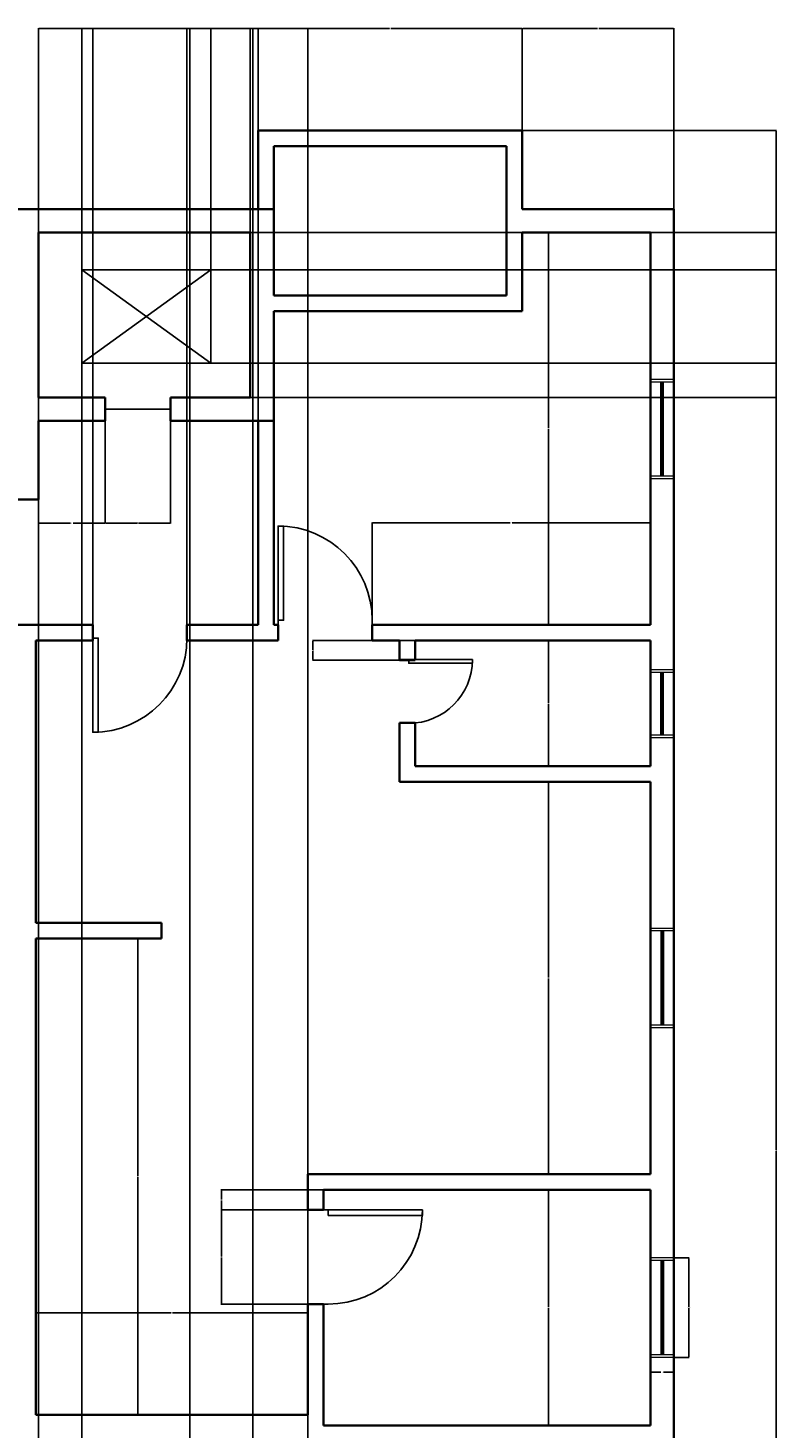
# Model space of a CAD drawing. Units: inches. Extents: x -7288 to -6705, y 7169 to 8028.
# Tile 5 of 5: x -6992 to -6705, y 7493 to 8028. Entities that reach past the tile are written whole.
import ezdxf

# ---------------------------------------------------------------- set-up
doc = ezdxf.new("R2010")
doc.units = ezdxf.units.IN
for name, color, linetype, lineweight in [('A-ANNO-DIMS', 2, 'Continuous', 18), ('A-DOOR', 3, 'Continuous', 25), ('A-FLOR-EVTR', 4, 'Continuous', 25), ('A-GLAZ', 2, 'Continuous', 18), ('A-WALL', 1, 'Continuous', 35)]:
    doc.layers.add(name, color=color, linetype=linetype, lineweight=lineweight)
doc.styles.get("Standard").update_dxf_attribs({"font": 'arial.ttf'})
doc.dimstyles.get("Standard").update_dxf_attribs({"dimtxt": 0.18, "dimasz": 0.18, "dimexe": 0.18, "dimexo": 0.0625, "dimgap": 0.09, "dimtad": 0, "dimtih": 1, "dimtoh": 1, "dimdec": 4, "dimzin": 0, "dimdsep": 46, "dimtxsty": 'Standard', "dimcen": 0.09, "dimadec": 0, "dimazin": 0, "dimtfac": 1, "dimtdec": 4, "dimtofl": 0, "dimtmove": 0, "dimatfit": 3, "dimfxl": 1, "dimtolj": 1, "dimtzin": 0, "dimarcsym": 0})

# ---------------------------------------------------------------- blocks, each defined once
blk = doc.blocks.new('*U8')
for p, q in [((0, 0), (0, -100)), ((750, 0), (750, -100))]:
    blk.add_line(p, q)
blk.add_lwpolyline([(0, 0), (0, 750), (43.75, 750), (43.75, 0)], close=True)
blk.add_arc((0, 0), 750, 0, 90)
blk = doc.blocks.new('WIN-36IN-WALL9')
for p, q in [((0, 38), (9, 38)), ((0, 37), (9, 37)), ((4, 1), (4, 37)), ((4.5, 1), (4.5, 37)), ((5, 1), (5, 37)), ((0, 1), (9, 1)), ((0, 0), (9, 0))]:
    blk.add_line(p, q)
blk = doc.blocks.new('WIN-24IN-WALL9')
for p, q in [((0, 26), (9, 26)), ((0, 25), (9, 25)), ((4, 1), (4, 25)), ((4.5, 1), (4.5, 25)), ((5, 1), (5, 25)), ((0, 1), (9, 1)), ((0, 0), (9, 0))]:
    blk.add_line(p, q)
blk = doc.blocks.new('*D87')
at = {"layer": 'A-ANNO-DIMS', "color": 0, "lineweight": -2, "transparency": 16777216}
for p, q in [((-6744.78, 7557.53), (-6738.96, 7557.53)), ((-6739.14, 7557.35), (-6739.14, 7538.71)), ((-6739.14, 7519.71), (-6739.14, 7538.35)), ((-6744.78, 7519.53), (-6738.96, 7519.53))]:
    blk.add_line(p, q, dxfattribs=at)
at = {"layer": 'A-ANNO-DIMS', "color": 0, "transparency": 16777216}
for points in [[(-6739.17, 7557.35), (-6739.11, 7557.35), (-6739.14, 7557.53)], [(-6739.17, 7519.71), (-6739.11, 7519.71), (-6739.14, 7519.53)]]:
    blk.add_solid(points, dxfattribs=at)
at = {"layer": 'Defpoints', "color": 0, "transparency": 16777216}
for p in [(-6744.84, 7557.53), (-6744.84, 7519.53), (-6739.14, 7519.53)]:
    blk.add_point(p, dxfattribs=at)
at = {"layer": 'A-ANNO-DIMS', "color": 0, "transparency": 16777216, "insert": (-6739.14, 7538.53), "char_height": 0.18, "attachment_point": 5}
blk.add_mtext('\\A1;W1 38 TYP.', dxfattribs=at)
blk = doc.blocks.new('*D88')
at = {"layer": 'A-ANNO-DIMS', "color": 0, "lineweight": -2, "transparency": 16777216}
for p, q in [((-6753.84, 7519.47), (-6753.84, 7513.65)), ((-6744.84, 7519.47), (-6744.84, 7513.65)), ((-6753.66, 7513.83), (-6749.8, 7513.83)), ((-6745.02, 7513.83), (-6748.88, 7513.83))]:
    blk.add_line(p, q, dxfattribs=at)
at = {"layer": 'A-ANNO-DIMS', "color": 0, "transparency": 16777216}
for points in [[(-6753.66, 7513.86), (-6753.66, 7513.8), (-6753.84, 7513.83)], [(-6745.02, 7513.86), (-6745.02, 7513.8), (-6744.84, 7513.83)]]:
    blk.add_solid(points, dxfattribs=at)
at = {"layer": 'Defpoints', "color": 0, "transparency": 16777216}
for p in [(-6753.84, 7519.53), (-6744.84, 7519.53), (-6753.84, 7513.83)]:
    blk.add_point(p, dxfattribs=at)
at = {"layer": 'A-ANNO-DIMS', "color": 0, "transparency": 16777216, "insert": (-6749.34, 7513.83), "char_height": 0.18, "attachment_point": 5}
blk.add_mtext('\\A1;9 TYP.', dxfattribs=at)
blk = doc.blocks.new('*D94')
at = {"layer": 'A-ANNO-DIMS', "color": 0, "lineweight": -2, "transparency": 16777216}
for p, q in [((-6802.78, 7988.53), (-6705.63, 7988.53)), ((-6705.81, 7988.35), (-6705.81, 7598.71)), ((-6705.81, 7208.71), (-6705.81, 7598.35)), ((-6744.78, 7208.53), (-6705.63, 7208.53))]:
    blk.add_line(p, q, dxfattribs=at)
at = {"layer": 'A-ANNO-DIMS', "color": 0, "transparency": 16777216}
for points in [[(-6705.84, 7988.35), (-6705.78, 7988.35), (-6705.81, 7988.53)], [(-6705.84, 7208.71), (-6705.78, 7208.71), (-6705.81, 7208.53)]]:
    blk.add_solid(points, dxfattribs=at)
at = {"layer": 'Defpoints', "color": 0, "transparency": 16777216}
for p in [(-6802.84, 7988.53), (-6705.81, 7988.53), (-6744.84, 7208.53)]:
    blk.add_point(p, dxfattribs=at)
at = {"layer": 'A-ANNO-DIMS', "color": 0, "transparency": 16777216, "insert": (-6705.81, 7598.53), "char_height": 0.18, "attachment_point": 5}
blk.add_mtext('\\A1;780', dxfattribs=at)
blk = doc.blocks.new('*D97')
at = {"layer": 'A-ANNO-DIMS', "color": 0, "lineweight": -2, "transparency": 16777216}
for p, q in [((-6903.84, 7988.59), (-6903.84, 8027.74)), ((-6903.66, 8027.56), (-6853.6, 8027.56)), ((-6803.02, 8027.56), (-6853.08, 8027.56)), ((-6802.84, 7988.59), (-6802.84, 8027.74))]:
    blk.add_line(p, q, dxfattribs=at)
at = {"layer": 'A-ANNO-DIMS', "color": 0, "transparency": 16777216}
for points in [[(-6903.66, 8027.59), (-6903.66, 8027.53), (-6903.84, 8027.56)], [(-6803.02, 8027.59), (-6803.02, 8027.53), (-6802.84, 8027.56)]]:
    blk.add_solid(points, dxfattribs=at)
at = {"layer": 'Defpoints', "color": 0, "transparency": 16777216}
for p in [(-6802.84, 8027.56), (-6903.84, 7988.53), (-6802.84, 7988.53)]:
    blk.add_point(p, dxfattribs=at)
at = {"layer": 'A-ANNO-DIMS', "color": 0, "transparency": 16777216, "insert": (-6853.34, 8027.56), "char_height": 0.18, "attachment_point": 5}
blk.add_mtext('\\A1;101', dxfattribs=at)
blk = doc.blocks.new('*D98')
at = {"layer": 'A-ANNO-DIMS', "color": 0, "lineweight": -2, "transparency": 16777216}
for p, q in [((-6802.84, 7988.59), (-6802.84, 8027.74)), ((-6802.66, 8027.56), (-6774.06, 8027.56)), ((-6745.02, 8027.56), (-6773.62, 8027.56)), ((-6744.84, 7958.59), (-6744.84, 8027.74))]:
    blk.add_line(p, q, dxfattribs=at)
at = {"layer": 'A-ANNO-DIMS', "color": 0, "transparency": 16777216}
for points in [[(-6802.66, 8027.59), (-6802.66, 8027.53), (-6802.84, 8027.56)], [(-6745.02, 8027.59), (-6745.02, 8027.53), (-6744.84, 8027.56)]]:
    blk.add_solid(points, dxfattribs=at)
at = {"layer": 'Defpoints', "color": 0, "transparency": 16777216}
for p in [(-6744.84, 8027.56), (-6802.84, 7988.53), (-6744.84, 7958.53)]:
    blk.add_point(p, dxfattribs=at)
at = {"layer": 'A-ANNO-DIMS', "color": 0, "transparency": 16777216, "insert": (-6773.84, 8027.56), "char_height": 0.18, "attachment_point": 5}
blk.add_mtext('\\A1;58', dxfattribs=at)
blk = doc.blocks.new('*D104')
at = {"layer": 'A-ANNO-DIMS', "color": 0, "lineweight": -2, "transparency": 16777216}
for p, q in [((-6987.84, 7949.59), (-6987.84, 8027.74)), ((-6987.66, 8027.56), (-6947.54, 8027.56)), ((-6907.02, 8027.56), (-6947.14, 8027.56)), ((-6906.84, 7949.59), (-6906.84, 8027.74))]:
    blk.add_line(p, q, dxfattribs=at)
at = {"layer": 'A-ANNO-DIMS', "color": 0, "transparency": 16777216}
for points in [[(-6987.66, 8027.59), (-6987.66, 8027.53), (-6987.84, 8027.56)], [(-6907.02, 8027.59), (-6907.02, 8027.53), (-6906.84, 8027.56)]]:
    blk.add_solid(points, dxfattribs=at)
at = {"layer": 'Defpoints', "color": 0, "transparency": 16777216}
for p in [(-6906.84, 8027.56), (-6987.84, 7949.53), (-6906.84, 7949.53)]:
    blk.add_point(p, dxfattribs=at)
at = {"layer": 'A-ANNO-DIMS', "color": 0, "transparency": 16777216, "insert": (-6947.34, 8027.56), "char_height": 0.18, "attachment_point": 5}
blk.add_mtext('\\A1;81', dxfattribs=at)
blk = doc.blocks.new('*D105')
at = {"layer": 'A-ANNO-DIMS', "color": 0, "lineweight": -2, "transparency": 16777216}
for p, q in [((-6906.78, 7949.53), (-6705.63, 7949.53)), ((-6705.81, 7949.35), (-6705.81, 7918.21)), ((-6705.81, 7886.71), (-6705.81, 7917.85)), ((-6906.78, 7886.53), (-6705.63, 7886.53))]:
    blk.add_line(p, q, dxfattribs=at)
at = {"layer": 'A-ANNO-DIMS', "color": 0, "transparency": 16777216}
for points in [[(-6705.84, 7949.35), (-6705.78, 7949.35), (-6705.81, 7949.53)], [(-6705.84, 7886.71), (-6705.78, 7886.71), (-6705.81, 7886.53)]]:
    blk.add_solid(points, dxfattribs=at)
at = {"layer": 'Defpoints', "color": 0, "transparency": 16777216}
for p in [(-6906.84, 7949.53), (-6705.81, 7949.53), (-6906.84, 7886.53)]:
    blk.add_point(p, dxfattribs=at)
at = {"layer": 'A-ANNO-DIMS', "color": 0, "transparency": 16777216, "insert": (-6705.81, 7918.03), "char_height": 0.18, "attachment_point": 5}
blk.add_mtext('\\A1;63', dxfattribs=at)
blk = doc.blocks.new('*D109')
at = {"layer": 'A-ANNO-DIMS', "color": 0, "lineweight": -2, "transparency": 16777216}
for p, q in [((-6962.28, 7877.47), (-6962.28, 7838.32)), ((-6937.29, 7877.47), (-6937.29, 7838.32)), ((-6962.1, 7838.5), (-6950.01, 7838.5)), ((-6937.47, 7838.5), (-6949.56, 7838.5))]:
    blk.add_line(p, q, dxfattribs=at)
at = {"layer": 'A-ANNO-DIMS', "color": 0, "transparency": 16777216}
for points in [[(-6962.1, 7838.53), (-6962.1, 7838.47), (-6962.28, 7838.5)], [(-6937.47, 7838.53), (-6937.47, 7838.47), (-6937.29, 7838.5)]]:
    blk.add_solid(points, dxfattribs=at)
at = {"layer": 'Defpoints', "color": 0, "transparency": 16777216}
for p in [(-6962.28, 7877.53), (-6937.29, 7877.53), (-6962.28, 7838.5)]:
    blk.add_point(p, dxfattribs=at)
at = {"layer": 'A-ANNO-DIMS', "color": 0, "transparency": 16777216, "insert": (-6949.78, 7838.5), "char_height": 0.18, "attachment_point": 5}
blk.add_mtext('\\A1;25', dxfattribs=at)
blk = doc.blocks.new('*D113')
at = {"layer": 'A-ANNO-DIMS', "color": 0, "lineweight": -2, "transparency": 16777216}
for p, q in [((-6971.26, 7935.37), (-6971.26, 8027.74)), ((-6971.08, 8027.56), (-6947.02, 8027.56)), ((-6922.15, 8027.56), (-6946.22, 8027.56)), ((-6921.97, 7935.37), (-6921.97, 8027.74))]:
    blk.add_line(p, q, dxfattribs=at)
at = {"layer": 'A-ANNO-DIMS', "color": 0, "transparency": 16777216}
for points in [[(-6971.08, 8027.59), (-6971.08, 8027.53), (-6971.26, 8027.56)], [(-6922.15, 8027.59), (-6922.15, 8027.53), (-6921.97, 8027.56)]]:
    blk.add_solid(points, dxfattribs=at)
at = {"layer": 'Defpoints', "color": 0, "transparency": 16777216}
for p in [(-6921.97, 8027.56), (-6971.26, 7935.31), (-6921.97, 7935.31)]:
    blk.add_point(p, dxfattribs=at)
at = {"layer": 'A-ANNO-DIMS', "color": 0, "transparency": 16777216, "insert": (-6946.62, 8027.56), "char_height": 0.18, "attachment_point": 5}
blk.add_mtext('\\A1;49.29', dxfattribs=at)
blk = doc.blocks.new('*D114')
at = {"layer": 'A-ANNO-DIMS', "color": 0, "lineweight": -2, "transparency": 16777216}
for p, q in [((-6921.91, 7935.31), (-6705.63, 7935.31)), ((-6705.81, 7935.13), (-6705.81, 7917.61)), ((-6705.81, 7899.73), (-6705.81, 7917.25)), ((-6921.91, 7899.55), (-6705.63, 7899.55))]:
    blk.add_line(p, q, dxfattribs=at)
at = {"layer": 'A-ANNO-DIMS', "color": 0, "transparency": 16777216}
for points in [[(-6705.84, 7935.13), (-6705.78, 7935.13), (-6705.81, 7935.31)], [(-6705.84, 7899.73), (-6705.78, 7899.73), (-6705.81, 7899.55)]]:
    blk.add_solid(points, dxfattribs=at)
at = {"layer": 'Defpoints', "color": 0, "transparency": 16777216}
for p in [(-6921.97, 7935.31), (-6705.81, 7935.31), (-6921.97, 7899.55)]:
    blk.add_point(p, dxfattribs=at)
at = {"layer": 'A-ANNO-DIMS', "color": 0, "transparency": 16777216, "insert": (-6705.81, 7917.43), "char_height": 0.18, "attachment_point": 5}
blk.add_mtext('\\A1;35.76', dxfattribs=at)
blk = doc.blocks.new('*D115')
at = {"layer": 'A-ANNO-DIMS', "color": 0, "lineweight": -2, "transparency": 16777216}
for p, q in [((-6971.26, 7899.49), (-6971.26, 7169.32)), ((-6987.84, 7886.47), (-6987.84, 7169.32)), ((-6987.66, 7169.5), (-6980.01, 7169.5)), ((-6971.44, 7169.5), (-6979.1, 7169.5))]:
    blk.add_line(p, q, dxfattribs=at)
at = {"layer": 'A-ANNO-DIMS', "color": 0, "transparency": 16777216}
for points in [[(-6987.66, 7169.53), (-6987.66, 7169.47), (-6987.84, 7169.5)], [(-6971.44, 7169.53), (-6971.44, 7169.47), (-6971.26, 7169.5)]]:
    blk.add_solid(points, dxfattribs=at)
at = {"layer": 'Defpoints', "color": 0, "transparency": 16777216}
for p in [(-6971.26, 7899.55), (-6987.84, 7886.53), (-6971.26, 7169.5)]:
    blk.add_point(p, dxfattribs=at)
at = {"layer": 'A-ANNO-DIMS', "color": 0, "transparency": 16777216, "insert": (-6979.55, 7169.5), "char_height": 0.18, "attachment_point": 5}
blk.add_mtext('\\A1;16.578', dxfattribs=at)
blk = doc.blocks.new('*D116')
at = {"layer": 'A-ANNO-DIMS', "color": 0, "lineweight": -2, "transparency": 16777216}
for p, q in [((-6987.78, 7949.53), (-6705.63, 7949.53)), ((-6705.81, 7949.35), (-6705.81, 7942.6)), ((-6705.81, 7935.49), (-6705.81, 7942.24)), ((-6971.2, 7935.31), (-6705.63, 7935.31))]:
    blk.add_line(p, q, dxfattribs=at)
at = {"layer": 'A-ANNO-DIMS', "color": 0, "transparency": 16777216}
for points in [[(-6705.84, 7949.35), (-6705.78, 7949.35), (-6705.81, 7949.53)], [(-6705.84, 7935.49), (-6705.78, 7935.49), (-6705.81, 7935.31)]]:
    blk.add_solid(points, dxfattribs=at)
at = {"layer": 'Defpoints', "color": 0, "transparency": 16777216}
for p in [(-6987.84, 7949.53), (-6705.81, 7949.53), (-6971.26, 7935.31)]:
    blk.add_point(p, dxfattribs=at)
at = {"layer": 'A-ANNO-DIMS', "color": 0, "transparency": 16777216, "insert": (-6705.81, 7942.42), "char_height": 0.18, "attachment_point": 5}
blk.add_mtext('\\A1;14.222', dxfattribs=at)
blk = doc.blocks.new('*D117')
at = {"layer": 'A-ANNO-DIMS', "color": 0, "lineweight": -2, "transparency": 16777216}
for p, q in [((-6987.84, 7877.47), (-6987.84, 7838.32)), ((-6962.28, 7877.47), (-6962.28, 7838.32)), ((-6987.66, 7838.5), (-6975.53, 7838.5)), ((-6962.46, 7838.5), (-6974.6, 7838.5))]:
    blk.add_line(p, q, dxfattribs=at)
at = {"layer": 'A-ANNO-DIMS', "color": 0, "transparency": 16777216}
for points in [[(-6987.66, 7838.53), (-6987.66, 7838.47), (-6987.84, 7838.5)], [(-6962.46, 7838.53), (-6962.46, 7838.47), (-6962.28, 7838.5)]]:
    blk.add_solid(points, dxfattribs=at)
at = {"layer": 'Defpoints', "color": 0, "transparency": 16777216}
for p in [(-6987.84, 7877.53), (-6962.28, 7877.53), (-6987.84, 7838.5)]:
    blk.add_point(p, dxfattribs=at)
at = {"layer": 'A-ANNO-DIMS', "color": 0, "transparency": 16777216, "insert": (-6975.06, 7838.5), "char_height": 0.18, "attachment_point": 5}
blk.add_mtext('\\A1;25.556', dxfattribs=at)
blk = doc.blocks.new('*D120')
at = {"layer": 'A-ANNO-DIMS', "color": 0, "lineweight": -2, "transparency": 16777216}
for p, q in [((-6967.07, 7799.59), (-6967.07, 8027.74)), ((-6966.89, 8027.56), (-6949.29, 8027.56)), ((-6931.25, 8027.56), (-6948.85, 8027.56)), ((-6931.07, 7799.59), (-6931.07, 8027.74))]:
    blk.add_line(p, q, dxfattribs=at)
at = {"layer": 'A-ANNO-DIMS', "color": 0, "transparency": 16777216}
for points in [[(-6966.89, 8027.59), (-6966.89, 8027.53), (-6967.07, 8027.56)], [(-6931.25, 8027.59), (-6931.25, 8027.53), (-6931.07, 8027.56)]]:
    blk.add_solid(points, dxfattribs=at)
at = {"layer": 'Defpoints', "color": 0, "transparency": 16777216}
for p in [(-6931.07, 8027.56), (-6967.07, 7799.53), (-6931.07, 7799.53)]:
    blk.add_point(p, dxfattribs=at)
at = {"layer": 'A-ANNO-DIMS', "color": 0, "transparency": 16777216, "insert": (-6949.07, 8027.56), "char_height": 0.18, "attachment_point": 5}
blk.add_mtext('\\A1;36', dxfattribs=at)
blk = doc.blocks.new('*D121')
at = {"layer": 'A-ANNO-DIMS', "color": 0, "lineweight": -2, "transparency": 16777216}
for p, q in [((-6931.07, 7799.59), (-6931.07, 8027.74)), ((-6930.89, 8027.56), (-6917.85, 8027.56)), ((-6904.02, 8027.56), (-6917.06, 8027.56)), ((-6903.84, 7799.59), (-6903.84, 8027.74))]:
    blk.add_line(p, q, dxfattribs=at)
at = {"layer": 'A-ANNO-DIMS', "color": 0, "transparency": 16777216}
for points in [[(-6930.89, 8027.59), (-6930.89, 8027.53), (-6931.07, 8027.56)], [(-6904.02, 8027.59), (-6904.02, 8027.53), (-6903.84, 8027.56)]]:
    blk.add_solid(points, dxfattribs=at)
at = {"layer": 'Defpoints', "color": 0, "transparency": 16777216}
for p in [(-6903.84, 8027.56), (-6931.07, 7799.53), (-6903.84, 7799.53)]:
    blk.add_point(p, dxfattribs=at)
at = {"layer": 'A-ANNO-DIMS', "color": 0, "transparency": 16777216, "insert": (-6917.45, 8027.56), "char_height": 0.18, "attachment_point": 5}
blk.add_mtext('\\A1;27.23', dxfattribs=at)
blk = doc.blocks.new('*D124')
at = {"layer": 'A-ANNO-DIMS', "color": 0, "lineweight": -2, "transparency": 16777216}
for p, q in [((-6860.23, 7799.59), (-6860.23, 7838.74)), ((-6860.05, 7838.56), (-6807.42, 7838.56)), ((-6754.02, 7838.56), (-6806.65, 7838.56)), ((-6753.84, 7799.59), (-6753.84, 7838.74))]:
    blk.add_line(p, q, dxfattribs=at)
at = {"layer": 'A-ANNO-DIMS', "color": 0, "transparency": 16777216}
for points in [[(-6860.05, 7838.59), (-6860.05, 7838.53), (-6860.23, 7838.56)], [(-6754.02, 7838.59), (-6754.02, 7838.53), (-6753.84, 7838.56)]]:
    blk.add_solid(points, dxfattribs=at)
at = {"layer": 'Defpoints', "color": 0, "transparency": 16777216}
for p in [(-6753.84, 7838.56), (-6860.23, 7799.53), (-6753.84, 7799.53)]:
    blk.add_point(p, dxfattribs=at)
at = {"layer": 'A-ANNO-DIMS', "color": 0, "transparency": 16777216, "insert": (-6807.04, 7838.56), "char_height": 0.18, "attachment_point": 5}
blk.add_mtext('\\A1;106.4', dxfattribs=at)
blk = doc.blocks.new('*D125')
at = {"layer": 'A-ANNO-DIMS', "color": 0, "lineweight": -2, "transparency": 16777216}
for p, q in [((-6753.9, 7949.53), (-6793.05, 7949.53)), ((-6792.87, 7949.35), (-6792.87, 7874.71)), ((-6792.87, 7799.71), (-6792.87, 7874.35)), ((-6753.9, 7799.53), (-6793.05, 7799.53))]:
    blk.add_line(p, q, dxfattribs=at)
at = {"layer": 'A-ANNO-DIMS', "color": 0, "transparency": 16777216}
for points in [[(-6792.9, 7949.35), (-6792.84, 7949.35), (-6792.87, 7949.53)], [(-6792.9, 7799.71), (-6792.84, 7799.71), (-6792.87, 7799.53)]]:
    blk.add_solid(points, dxfattribs=at)
at = {"layer": 'Defpoints', "color": 0, "transparency": 16777216}
for p in [(-6792.87, 7949.53), (-6753.84, 7949.53), (-6753.84, 7799.53)]:
    blk.add_point(p, dxfattribs=at)
at = {"layer": 'A-ANNO-DIMS', "color": 0, "transparency": 16777216, "insert": (-6792.87, 7874.53), "char_height": 0.18, "attachment_point": 5}
blk.add_mtext('\\A1;150', dxfattribs=at)
blk = doc.blocks.new('*D128')
at = {"layer": 'A-ANNO-DIMS', "color": 0, "lineweight": -2, "transparency": 16777216}
for p, q in [((-6753.9, 7793.53), (-6793.05, 7793.53)), ((-6792.87, 7793.35), (-6792.87, 7769.71)), ((-6792.87, 7745.71), (-6792.87, 7769.35)), ((-6753.9, 7745.53), (-6793.05, 7745.53))]:
    blk.add_line(p, q, dxfattribs=at)
at = {"layer": 'A-ANNO-DIMS', "color": 0, "transparency": 16777216}
for points in [[(-6792.9, 7793.35), (-6792.84, 7793.35), (-6792.87, 7793.53)], [(-6792.9, 7745.71), (-6792.84, 7745.71), (-6792.87, 7745.53)]]:
    blk.add_solid(points, dxfattribs=at)
at = {"layer": 'Defpoints', "color": 0, "transparency": 16777216}
for p in [(-6792.87, 7793.53), (-6753.84, 7793.53), (-6753.84, 7745.53)]:
    blk.add_point(p, dxfattribs=at)
at = {"layer": 'A-ANNO-DIMS', "color": 0, "transparency": 16777216, "insert": (-6792.87, 7769.53), "char_height": 0.18, "attachment_point": 5}
blk.add_mtext('\\A1;48', dxfattribs=at)
blk = doc.blocks.new('*D130')
at = {"layer": 'A-ANNO-DIMS', "color": 0, "lineweight": -2, "transparency": 16777216}
for p, q in [((-6843.9, 7793.53), (-6883.05, 7793.53)), ((-6882.87, 7793.35), (-6882.87, 7790)), ((-6882.87, 7786.29), (-6882.87, 7789.64)), ((-6843.9, 7786.11), (-6883.05, 7786.11))]:
    blk.add_line(p, q, dxfattribs=at)
at = {"layer": 'A-ANNO-DIMS', "color": 0, "transparency": 16777216}
for points in [[(-6882.9, 7793.35), (-6882.84, 7793.35), (-6882.87, 7793.53)], [(-6882.9, 7786.29), (-6882.84, 7786.29), (-6882.87, 7786.11)]]:
    blk.add_solid(points, dxfattribs=at)
at = {"layer": 'Defpoints', "color": 0, "transparency": 16777216}
for p in [(-6882.87, 7793.53), (-6843.84, 7793.53), (-6843.84, 7786.11)]:
    blk.add_point(p, dxfattribs=at)
at = {"layer": 'A-ANNO-DIMS', "color": 0, "transparency": 16777216, "insert": (-6882.87, 7789.82), "char_height": 0.18, "attachment_point": 5}
blk.add_mtext('\\A1;7.424', dxfattribs=at)
blk = doc.blocks.new('*D132')
at = {"layer": 'A-ANNO-DIMS', "color": 0, "lineweight": -2, "transparency": 16777216}
for p, q in [((-6988.84, 7497.59), (-6988.84, 7536.74)), ((-6988.66, 7536.56), (-6937.12, 7536.56)), ((-6885.02, 7536.56), (-6936.56, 7536.56)), ((-6884.84, 7497.59), (-6884.84, 7536.74))]:
    blk.add_line(p, q, dxfattribs=at)
at = {"layer": 'A-ANNO-DIMS', "color": 0, "transparency": 16777216}
for points in [[(-6988.66, 7536.59), (-6988.66, 7536.53), (-6988.84, 7536.56)], [(-6885.02, 7536.59), (-6885.02, 7536.53), (-6884.84, 7536.56)]]:
    blk.add_solid(points, dxfattribs=at)
at = {"layer": 'Defpoints', "color": 0, "transparency": 16777216}
for p in [(-6884.84, 7536.56), (-6988.84, 7497.53), (-6884.84, 7497.53)]:
    blk.add_point(p, dxfattribs=at)
at = {"layer": 'A-ANNO-DIMS', "color": 0, "transparency": 16777216, "insert": (-6936.84, 7536.56), "char_height": 0.18, "attachment_point": 5}
blk.add_mtext('\\A1;104', dxfattribs=at)
blk = doc.blocks.new('*D133')
at = {"layer": 'A-ANNO-DIMS', "color": 0, "lineweight": -2, "transparency": 16777216}
for p, q in [((-6753.9, 7739.53), (-6793.05, 7739.53)), ((-6792.87, 7739.35), (-6792.87, 7664.71)), ((-6792.87, 7589.71), (-6792.87, 7664.35)), ((-6753.9, 7589.53), (-6793.05, 7589.53))]:
    blk.add_line(p, q, dxfattribs=at)
at = {"layer": 'A-ANNO-DIMS', "color": 0, "transparency": 16777216}
for points in [[(-6792.9, 7739.35), (-6792.84, 7739.35), (-6792.87, 7739.53)], [(-6792.9, 7589.71), (-6792.84, 7589.71), (-6792.87, 7589.53)]]:
    blk.add_solid(points, dxfattribs=at)
at = {"layer": 'Defpoints', "color": 0, "transparency": 16777216}
for p in [(-6792.87, 7739.53), (-6753.84, 7739.53), (-6753.84, 7589.53)]:
    blk.add_point(p, dxfattribs=at)
at = {"layer": 'A-ANNO-DIMS', "color": 0, "transparency": 16777216, "insert": (-6792.87, 7664.53), "char_height": 0.18, "attachment_point": 5}
blk.add_mtext('\\A1;150', dxfattribs=at)
blk = doc.blocks.new('*D136')
at = {"layer": 'A-ANNO-DIMS', "color": 0, "lineweight": -2, "transparency": 16777216}
for p, q in [((-6988.78, 7679.64), (-6949.63, 7679.64)), ((-6949.81, 7679.46), (-6949.81, 7588.77)), ((-6949.81, 7497.71), (-6949.81, 7588.4)), ((-6988.78, 7497.53), (-6949.63, 7497.53))]:
    blk.add_line(p, q, dxfattribs=at)
at = {"layer": 'A-ANNO-DIMS', "color": 0, "transparency": 16777216}
for points in [[(-6949.84, 7679.46), (-6949.78, 7679.46), (-6949.81, 7679.64)], [(-6949.84, 7497.71), (-6949.78, 7497.71), (-6949.81, 7497.53)]]:
    blk.add_solid(points, dxfattribs=at)
at = {"layer": 'Defpoints', "color": 0, "transparency": 16777216}
for p in [(-6988.84, 7679.64), (-6988.84, 7497.53), (-6949.81, 7497.53)]:
    blk.add_point(p, dxfattribs=at)
at = {"layer": 'A-ANNO-DIMS', "color": 0, "transparency": 16777216, "insert": (-6949.81, 7588.59), "char_height": 0.18, "attachment_point": 5}
blk.add_mtext('\\A1;182.1', dxfattribs=at)
blk = doc.blocks.new('*D138')
at = {"layer": 'A-ANNO-DIMS', "color": 0, "lineweight": -2, "transparency": 16777216}
for p, q in [((-6753.9, 7583.53), (-6793.05, 7583.53)), ((-6792.87, 7583.35), (-6792.87, 7538.71)), ((-6792.87, 7493.71), (-6792.87, 7538.35)), ((-6753.9, 7493.53), (-6793.05, 7493.53))]:
    blk.add_line(p, q, dxfattribs=at)
at = {"layer": 'A-ANNO-DIMS', "color": 0, "transparency": 16777216}
for points in [[(-6792.9, 7583.35), (-6792.84, 7583.35), (-6792.87, 7583.53)], [(-6792.9, 7493.71), (-6792.84, 7493.71), (-6792.87, 7493.53)]]:
    blk.add_solid(points, dxfattribs=at)
at = {"layer": 'Defpoints', "color": 0, "transparency": 16777216}
for p in [(-6792.87, 7583.53), (-6753.84, 7583.53), (-6753.84, 7493.53)]:
    blk.add_point(p, dxfattribs=at)
at = {"layer": 'A-ANNO-DIMS', "color": 0, "transparency": 16777216, "insert": (-6792.87, 7538.53), "char_height": 0.18, "attachment_point": 5}
blk.add_mtext('\\A1;90', dxfattribs=at)
blk = doc.blocks.new('*D154')
at = {"layer": 'A-ANNO-DIMS', "color": 0, "lineweight": -2, "transparency": 16777216}
for p, q in [((-6905.9, 7347.59), (-6905.9, 8027.74)), ((-6905.72, 8027.56), (-6895.77, 8027.56)), ((-6885.02, 8027.56), (-6894.97, 8027.56)), ((-6884.84, 7347.59), (-6884.84, 8027.74))]:
    blk.add_line(p, q, dxfattribs=at)
at = {"layer": 'A-ANNO-DIMS', "color": 0, "transparency": 16777216}
for points in [[(-6905.72, 8027.59), (-6905.72, 8027.53), (-6905.9, 8027.56)], [(-6885.02, 8027.59), (-6885.02, 8027.53), (-6884.84, 8027.56)]]:
    blk.add_solid(points, dxfattribs=at)
at = {"layer": 'Defpoints', "color": 0, "transparency": 16777216}
for p in [(-6884.84, 8027.56), (-6905.9, 7347.53), (-6884.84, 7347.53)]:
    blk.add_point(p, dxfattribs=at)
at = {"layer": 'A-ANNO-DIMS', "color": 0, "transparency": 16777216, "insert": (-6895.37, 8027.56), "char_height": 0.18, "attachment_point": 5}
blk.add_mtext('\\A1;21.06', dxfattribs=at)
blk = doc.blocks.new('*D155')
at = {"layer": 'A-ANNO-DIMS', "color": 0, "lineweight": -2, "transparency": 16777216}
for p, q in [((-6929.9, 7347.59), (-6929.9, 8027.74)), ((-6929.72, 8027.56), (-6918.12, 8027.56)), ((-6906.08, 8027.56), (-6917.68, 8027.56)), ((-6905.9, 7347.59), (-6905.9, 8027.74))]:
    blk.add_line(p, q, dxfattribs=at)
at = {"layer": 'A-ANNO-DIMS', "color": 0, "transparency": 16777216}
for points in [[(-6929.72, 8027.59), (-6929.72, 8027.53), (-6929.9, 8027.56)], [(-6906.08, 8027.59), (-6906.08, 8027.53), (-6905.9, 8027.56)]]:
    blk.add_solid(points, dxfattribs=at)
at = {"layer": 'Defpoints', "color": 0, "transparency": 16777216}
for p in [(-6905.9, 8027.56), (-6929.9, 7347.53), (-6905.9, 7347.53)]:
    blk.add_point(p, dxfattribs=at)
at = {"layer": 'A-ANNO-DIMS', "color": 0, "transparency": 16777216, "insert": (-6917.9, 8027.56), "char_height": 0.18, "attachment_point": 5}
blk.add_mtext('\\A1;24', dxfattribs=at)
blk = doc.blocks.new('*D163')
at = {"layer": 'A-ANNO-DIMS', "color": 0, "lineweight": -2, "transparency": 16777216}
for p, q in [((-6878.9, 7575.9), (-6918.05, 7575.9)), ((-6917.87, 7575.72), (-6917.87, 7558.08)), ((-6917.87, 7540.08), (-6917.87, 7557.72)), ((-6878.9, 7539.9), (-6918.05, 7539.9))]:
    blk.add_line(p, q, dxfattribs=at)
at = {"layer": 'A-ANNO-DIMS', "color": 0, "transparency": 16777216}
for points in [[(-6917.9, 7575.72), (-6917.84, 7575.72), (-6917.87, 7575.9)], [(-6917.9, 7540.08), (-6917.84, 7540.08), (-6917.87, 7539.9)]]:
    blk.add_solid(points, dxfattribs=at)
at = {"layer": 'Defpoints', "color": 0, "transparency": 16777216}
for p in [(-6917.87, 7575.9), (-6878.84, 7575.9), (-6878.84, 7539.9)]:
    blk.add_point(p, dxfattribs=at)
at = {"layer": 'A-ANNO-DIMS', "color": 0, "transparency": 16777216, "insert": (-6917.87, 7557.9), "char_height": 0.18, "attachment_point": 5}
blk.add_mtext('\\A1;36', dxfattribs=at)
blk = doc.blocks.new('*D166')
at = {"layer": 'A-ANNO-DIMS', "color": 0, "lineweight": -2, "transparency": 16777216}
for p, q in [((-6878.9, 7583.53), (-6918.05, 7583.53)), ((-6917.87, 7583.35), (-6917.87, 7579.9)), ((-6917.87, 7576.08), (-6917.87, 7579.53)), ((-6878.9, 7575.9), (-6918.05, 7575.9))]:
    blk.add_line(p, q, dxfattribs=at)
at = {"layer": 'A-ANNO-DIMS', "color": 0, "transparency": 16777216}
for points in [[(-6917.9, 7583.35), (-6917.84, 7583.35), (-6917.87, 7583.53)], [(-6917.9, 7576.08), (-6917.84, 7576.08), (-6917.87, 7575.9)]]:
    blk.add_solid(points, dxfattribs=at)
at = {"layer": 'Defpoints', "color": 0, "transparency": 16777216}
for p in [(-6917.87, 7583.53), (-6878.84, 7583.53), (-6878.84, 7575.9)]:
    blk.add_point(p, dxfattribs=at)
at = {"layer": 'A-ANNO-DIMS', "color": 0, "transparency": 16777216, "insert": (-6917.87, 7579.72), "char_height": 0.18, "attachment_point": 5}
blk.add_mtext('\\A1;7.63', dxfattribs=at)

msp = doc.modelspace()

# ---------------------------------------------------------------- linework, layer by layer
at = {"layer": 'A-FLOR-EVTR'}
for p, q in [((-6971.2622, 7935.3093), (-6921.9742, 7935.3093)), ((-6971.2622, 7899.5515), (-6971.2622, 7935.3093)), ((-6921.9742, 7935.3093), (-6971.2622, 7899.5515)), ((-6971.2622, 7935.3093), (-6921.9742, 7899.5515)), ((-6921.9742, 7935.3093), (-6921.9742, 7899.5515)), ((-6921.9742, 7899.5515), (-6971.2622, 7899.5515)), ((-6962.2837, 7882.0311), (-6937.2854, 7882.0311))]:
    msp.add_line(p, q, dxfattribs=at)
at = {"layer": 'A-WALL'}
for p, q in [((-6903.8398, 7988.5311), (-6903.8398, 7958.5311)), ((-6903.8398, 7988.5311), (-6802.8398, 7988.5311)), ((-6802.8398, 7988.5311), (-6802.8398, 7958.5311)), ((-6897.8398, 7982.5311), (-6897.8398, 7925.5311)), ((-6897.8398, 7982.5311), (-6808.8398, 7982.5311)), ((-6897.8398, 7982.5311), (-6897.8398, 7925.5311)), ((-6808.8398, 7982.5311), (-6808.8398, 7925.5311)), ((-7095.8398, 7958.5311), (-6897.8398, 7958.5311)), ((-6802.8398, 7958.5311), (-6744.8398, 7958.5311)), ((-6744.8398, 7958.5311), (-6744.8398, 7208.5311)), ((-6987.8398, 7949.5311), (-6987.8398, 7886.5311)), ((-6987.8398, 7949.5311), (-6906.8398, 7949.5311)), ((-6906.8398, 7949.5311), (-6906.8398, 7886.5311)), ((-6802.8398, 7949.5311), (-6753.8398, 7949.5311)), ((-6802.8398, 7949.5311), (-6802.8398, 7919.5311)), ((-6753.8398, 7949.5311), (-6753.8398, 7799.5311)), ((-6897.8398, 7925.5311), (-6808.8398, 7925.5311)), ((-6897.8398, 7919.5311), (-6802.8398, 7919.5311)), ((-6897.8398, 7919.5311), (-6897.8398, 7799.5311)), ((-6897.8398, 7919.5311), (-6897.8398, 7799.5311)), ((-6987.8398, 7886.5311), (-6962.2837, 7886.5311)), ((-6962.2837, 7886.5311), (-6962.2837, 7877.5311)), ((-6937.2854, 7886.5311), (-6937.2854, 7877.5311)), ((-6937.2854, 7886.5311), (-6906.8398, 7886.5311)), ((-6987.8398, 7877.5311), (-6962.2837, 7877.5311)), ((-6987.8398, 7877.5311), (-6987.8398, 7847.5311)), ((-6937.2854, 7877.5311), (-6897.8398, 7877.5311)), ((-6903.8398, 7877.5311), (-6903.8398, 7799.5311)), ((-6987.8398, 7847.5311), (-6996.8398, 7847.5311)), ((-7023.607, 7799.5311), (-6967.0693, 7799.5311)), ((-6967.0693, 7799.5311), (-6967.0693, 7793.5311)), ((-6931.0693, 7799.5311), (-6931.0693, 7793.5311)), ((-6931.0693, 7799.5311), (-6903.8398, 7799.5311)), ((-6897.8398, 7799.5311), (-6896.2321, 7799.5311)), ((-6896.2321, 7799.5311), (-6896.2321, 7793.5311)), ((-6860.2321, 7799.5311), (-6860.2321, 7793.5311)), ((-6860.2321, 7799.5311), (-6753.8398, 7799.5311)), ((-6988.8398, 7685.639), (-6988.8398, 7793.5311)), ((-6988.8398, 7793.5311), (-6967.0693, 7793.5311)), ((-6931.0693, 7793.5311), (-6896.2321, 7793.5311)), ((-6860.2321, 7793.5311), (-6849.8398, 7793.5311)), ((-6849.8398, 7793.5311), (-6849.8398, 7786.1066)), ((-6843.8398, 7793.5311), (-6843.8398, 7786.1066)), ((-6843.8398, 7793.5311), (-6753.8398, 7793.5311)), ((-6753.8398, 7793.5311), (-6753.8398, 7745.5311)), ((-6849.8398, 7786.1066), (-6843.8398, 7786.1066)), ((-6849.8398, 7762.1066), (-6843.8398, 7762.1066)), ((-6849.8398, 7762.1066), (-6849.8398, 7739.5311)), ((-6843.8398, 7762.1066), (-6843.8398, 7745.5311)), ((-6843.8398, 7745.5311), (-6753.8398, 7745.5311)), ((-6849.8398, 7739.5311), (-6753.8398, 7739.5311)), ((-6753.8398, 7739.5311), (-6753.8398, 7589.5311)), ((-6988.8398, 7685.639), (-6940.8398, 7685.639)), ((-6940.8398, 7685.639), (-6940.8398, 7679.639)), ((-6940.8398, 7679.639), (-6988.8398, 7679.639)), ((-6988.8398, 7497.5311), (-6988.8398, 7679.639)), ((-6884.8398, 7589.5311), (-6753.8398, 7589.5311)), ((-6884.8398, 7589.5311), (-6884.8398, 7575.9018)), ((-6878.8398, 7583.5311), (-6753.8398, 7583.5311)), ((-6878.8398, 7583.5311), (-6878.8398, 7575.9018)), ((-6753.8398, 7583.5311), (-6753.8398, 7493.5311)), ((-6884.8398, 7575.9018), (-6878.8398, 7575.9018)), ((-6884.8398, 7539.9018), (-6878.8398, 7539.9018)), ((-6884.8398, 7539.9018), (-6884.8398, 7497.5311)), ((-6878.8398, 7539.9018), (-6878.8398, 7493.5311)), ((-6884.8398, 7497.5311), (-6988.8398, 7497.5311)), ((-6878.8398, 7493.5311), (-6753.8398, 7493.5311))]:
    msp.add_line(p, q, dxfattribs=at)

# ---------------------------------------------------------------- block references
at = {"layer": 'A-DOOR', "xscale": 0.0479999999999998, "yscale": 0.0479999999999998, "zscale": 0.0479999999999998}
msp.add_blockref('*U8', (-6896.2321, 7801.3311), dxfattribs=at)
at = {"layer": 'A-DOOR'}
for p, xscale, yscale, zscale, rotation in [((-6967.0857, 7794.5267), -0.0480219550003032, 0.0480219550003032, 0.0480219550003032, 180), ((-6846.2473, 7786.2918), 0.0324798355098664, 0.0324798355098664, 0.0324798355098664, 270), ((-6877.0398, 7575.9018), 0.0479999962848893, 0.0479999962848893, 0.0479999962848893, 270)]:
    msp.add_blockref('*U8', p, dxfattribs=dict(at, xscale=xscale, yscale=yscale, zscale=zscale, rotation=rotation))
at = {"layer": 'A-GLAZ'}
for name, p in [('WIN-36IN-WALL9', (-6753.8398, 7855.5311)), ('WIN-24IN-WALL9', (-6753.8398, 7756.5311))]:
    msp.add_blockref(name, p, dxfattribs=at)
at = {"layer": 'A-GLAZ', "rotation": 180}
for p in [(-6744.8398, 7683.5311), (-6744.8398, 7557.5311)]:
    msp.add_blockref('WIN-36IN-WALL9', p, dxfattribs=at)

# ---------------------------------------------------------------- dimensions: what is measured, and where the dimension line sits
at = {"layer": 'A-ANNO-DIMS'}
for base, p1, p2, override, picture, middle in [((-6906.8398, 8027.5611), (-6987.8398, 7949.5311), (-6906.8398, 7949.5311), {"dimdec": 0, "dimlfac": 1, "dimrnd": 0, "dimzin": 0, "dimdsep": 46, "dimlunit": 2}, '*D104', (-6947.3398, 8027.5611)), ((-6921.9742, 8027.5611), (-6971.2622, 7935.3093), (-6921.9742, 7935.3093), {"dimdec": 2, "dimlfac": 1, "dimrnd": 0, "dimzin": 0, "dimdsep": 46, "dimlunit": 2}, '*D113', (-6946.6182, 8027.5611)), ((-6931.0693, 8027.5611), (-6967.0693, 7799.5311), (-6931.0693, 7799.5311), {"dimdec": 0, "dimlfac": 1, "dimrnd": 0, "dimzin": 0, "dimdsep": 46, "dimlunit": 2}, '*D120', (-6949.0693, 8027.5611)), ((-6903.8398, 8027.5611), (-6931.0693, 7799.5311), (-6903.8398, 7799.5311), {"dimdec": 2, "dimlfac": 1, "dimrnd": 0, "dimzin": 0, "dimdsep": 46, "dimlunit": 2}, '*D121', (-6917.4545, 8027.5611)), ((-6905.9003, 8027.5611), (-6929.9003, 7347.5311), (-6905.9003, 7347.5311), {"dimdec": 0, "dimlfac": 1, "dimrnd": 0, "dimzin": 0, "dimdsep": 46, "dimlunit": 2}, '*D155', (-6917.9003, 8027.5611)), ((-6884.8398, 8027.5611), (-6905.9003, 7347.5311), (-6884.8398, 7347.5311), {"dimdec": 2, "dimlfac": 1, "dimrnd": 0, "dimzin": 0, "dimdsep": 46, "dimlunit": 2}, '*D154', (-6895.3701, 8027.5611)), ((-6802.8398, 8027.5611), (-6903.8398, 7988.5311), (-6802.8398, 7988.5311), {"dimdec": 0, "dimlfac": 1, "dimrnd": 0, "dimzin": 0, "dimdsep": 46, "dimlunit": 2}, '*D97', (-6853.3398, 8027.5611)), ((-6744.8398, 8027.5611), (-6802.8398, 7988.5311), (-6744.8398, 7958.5311), {"dimdec": 0, "dimlfac": 1, "dimrnd": 0, "dimzin": 0, "dimdsep": 46, "dimlunit": 2}, '*D98', (-6773.8398, 8027.5611)), ((-6971.2622, 7169.5011), (-6987.8398, 7886.5311), (-6971.2622, 7899.5515), {"dimdec": 3, "dimlfac": 1, "dimrnd": 0, "dimzin": 0, "dimdsep": 46, "dimlunit": 2}, '*D115', (-6979.551, 7169.5011)), ((-6753.8398, 7838.5611), (-6860.2321, 7799.5311), (-6753.8398, 7799.5311), {"dimdec": 1, "dimlfac": 1, "dimrnd": 0, "dimzin": 0, "dimdsep": 46, "dimlunit": 2}, '*D124', (-6807.036, 7838.5611)), ((-6884.8398, 7536.5611), (-6988.8398, 7497.5311), (-6884.8398, 7497.5311), {"dimdec": 0, "dimlfac": 1, "dimrnd": 0, "dimzin": 0, "dimdsep": 46, "dimlunit": 2}, '*D132', (-6936.8398, 7536.5611))]:
    dim = msp.add_linear_dim(base=base, p1=p1, p2=p2, dimstyle='Standard', override=override, dxfattribs=at)
    dim.commit()
    dim.dimension.update_dxf_attribs({"geometry": picture, "text_midpoint": middle})
for base, p1, p2, angle, override, picture, middle in [((-6705.8098, 7988.5311), (-6744.8398, 7208.5311), (-6802.8398, 7988.5311), 90, {"dimdec": 0, "dimlfac": 1, "dimrnd": 0, "dimzin": 0, "dimdsep": 46, "dimlunit": 2}, '*D94', (-6705.8098, 7598.5311)), ((-6705.8098, 7949.5311), (-6971.2622, 7935.3093), (-6987.8398, 7949.5311), 90, {"dimdec": 3, "dimlfac": 1, "dimrnd": 0, "dimzin": 0, "dimdsep": 46, "dimlunit": 2}, '*D116', (-6705.8098, 7942.4202)), ((-6705.8098, 7949.5311), (-6906.8398, 7886.5311), (-6906.8398, 7949.5311), 90, {"dimdec": 0, "dimlfac": 1, "dimrnd": 0, "dimzin": 0, "dimdsep": 46, "dimlunit": 2}, '*D105', (-6705.8098, 7918.0311)), ((-6792.8698, 7949.5311), (-6753.8398, 7799.5311), (-6753.8398, 7949.5311), 90, {"dimdec": 0, "dimlfac": 1, "dimrnd": 0, "dimzin": 0, "dimdsep": 46, "dimlunit": 2}, '*D125', (-6792.8698, 7874.5311)), ((-6705.8098, 7935.3093), (-6921.9742, 7899.5515), (-6921.9742, 7935.3093), 90, {"dimdec": 2, "dimlfac": 1, "dimrnd": 0, "dimzin": 0, "dimdsep": 46, "dimlunit": 2}, '*D114', (-6705.8098, 7917.4304)), ((-6987.8398, 7838.5011), (-6962.2837, 7877.5311), (-6987.8398, 7877.5311), 180, {"dimdec": 3, "dimlfac": 1, "dimrnd": 0, "dimzin": 0, "dimdsep": 46, "dimlunit": 2}, '*D117', (-6975.0617, 7838.5011)), ((-6962.2837, 7838.5011), (-6937.2854, 7877.5311), (-6962.2837, 7877.5311), 180, {"dimdec": 0, "dimlfac": 1, "dimrnd": 0, "dimzin": 0, "dimdsep": 46, "dimlunit": 2}, '*D109', (-6949.7845, 7838.5011)), ((-6882.86982, 7793.5311), (-6843.83981, 7786.10661), (-6843.83981, 7793.5311), 90, {"dimdec": 3, "dimlfac": 1, "dimrnd": 0, "dimzin": 0, "dimdsep": 46, "dimlunit": 2}, '*D130', (-6882.86982, 7789.81886)), ((-6792.8698, 7793.5311), (-6753.8398, 7745.5311), (-6753.8398, 7793.5311), 90, {"dimdec": 0, "dimlfac": 1, "dimrnd": 0, "dimzin": 0, "dimdsep": 46, "dimlunit": 2}, '*D128', (-6792.8698, 7769.5311)), ((-6792.8698, 7739.5311), (-6753.8398, 7589.5311), (-6753.8398, 7739.5311), 90, {"dimdec": 0, "dimlfac": 1, "dimrnd": 0, "dimzin": 0, "dimdsep": 46, "dimlunit": 2}, '*D133', (-6792.8698, 7664.5311)), ((-6949.8098, 7497.5311), (-6988.8398, 7679.639), (-6988.8398, 7497.5311), 270, {"dimdec": 1, "dimlfac": 1, "dimrnd": 0, "dimzin": 0, "dimdsep": 46, "dimlunit": 2}, '*D136', (-6949.8098, 7588.585)), ((-6917.8698, 7583.5311), (-6878.8398, 7575.9018), (-6878.8398, 7583.5311), 90, {"dimdec": 2, "dimlfac": 1, "dimrnd": 0, "dimzin": 0, "dimdsep": 46, "dimlunit": 2}, '*D166', (-6917.8698, 7579.7164)), ((-6792.8698, 7583.5311), (-6753.8398, 7493.5311), (-6753.8398, 7583.5311), 90, {"dimdec": 0, "dimlfac": 1, "dimrnd": 0, "dimzin": 0, "dimdsep": 46, "dimlunit": 2}, '*D138', (-6792.8698, 7538.5311)), ((-6917.8698, 7575.9018), (-6878.8398, 7539.9018), (-6878.8398, 7575.9018), 90, {"dimdec": 0, "dimlfac": 1, "dimrnd": 0, "dimzin": 0, "dimdsep": 46, "dimlunit": 2}, '*D163', (-6917.8698, 7557.9018))]:
    dim = msp.add_linear_dim(base=base, p1=p1, p2=p2, angle=angle, dimstyle='Standard', override=override, dxfattribs=at)
    dim.commit()
    dim.dimension.update_dxf_attribs({"geometry": picture, "text_midpoint": middle})
for base, p1, p2, angle, text, picture, middle in [((-6739.1398, 7519.5311), (-6744.8398, 7557.5311), (-6744.8398, 7519.5311), 270, 'W1 <> TYP.', '*D87', (-6739.1398, 7538.5311)), ((-6753.8398, 7513.8311), (-6744.8398, 7519.5311), (-6753.8398, 7519.5311), 180, '<> TYP.', '*D88', (-6749.3398, 7513.8311))]:
    dim = msp.add_linear_dim(base=base, p1=p1, p2=p2, angle=angle, text=text, dimstyle='Standard', override={"dimdec": 0, "dimlfac": 1, "dimrnd": 0, "dimzin": 0, "dimdsep": 46, "dimlunit": 2}, dxfattribs=at)
    dim.commit()
    dim.dimension.update_dxf_attribs({"geometry": picture, "text_midpoint": middle})

doc.saveas('drawing.dxf')
